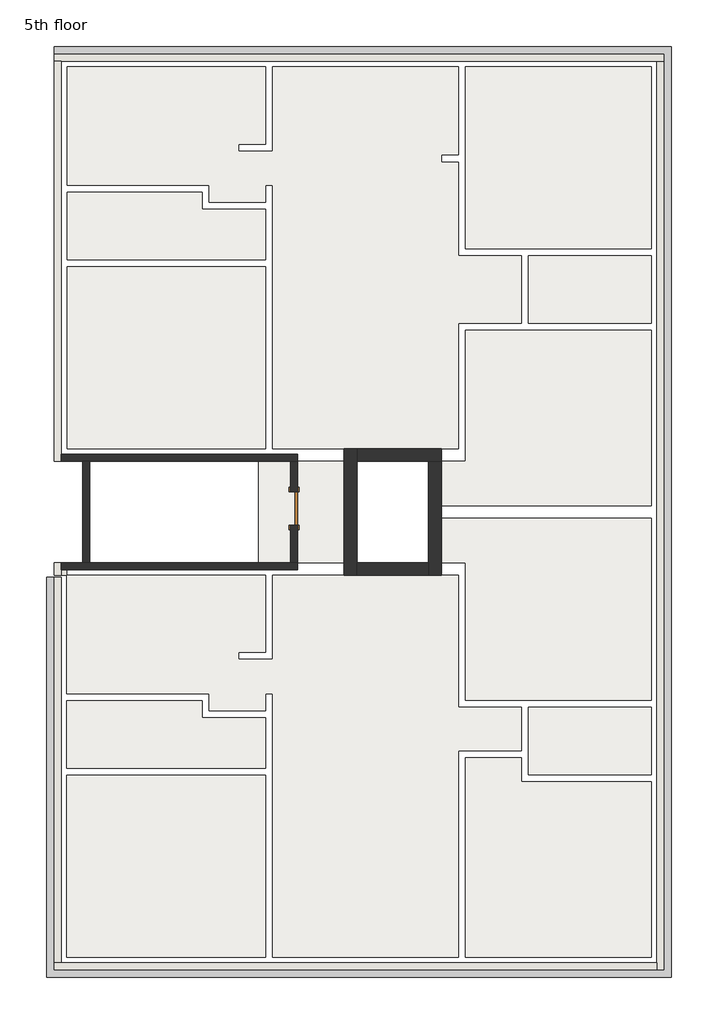
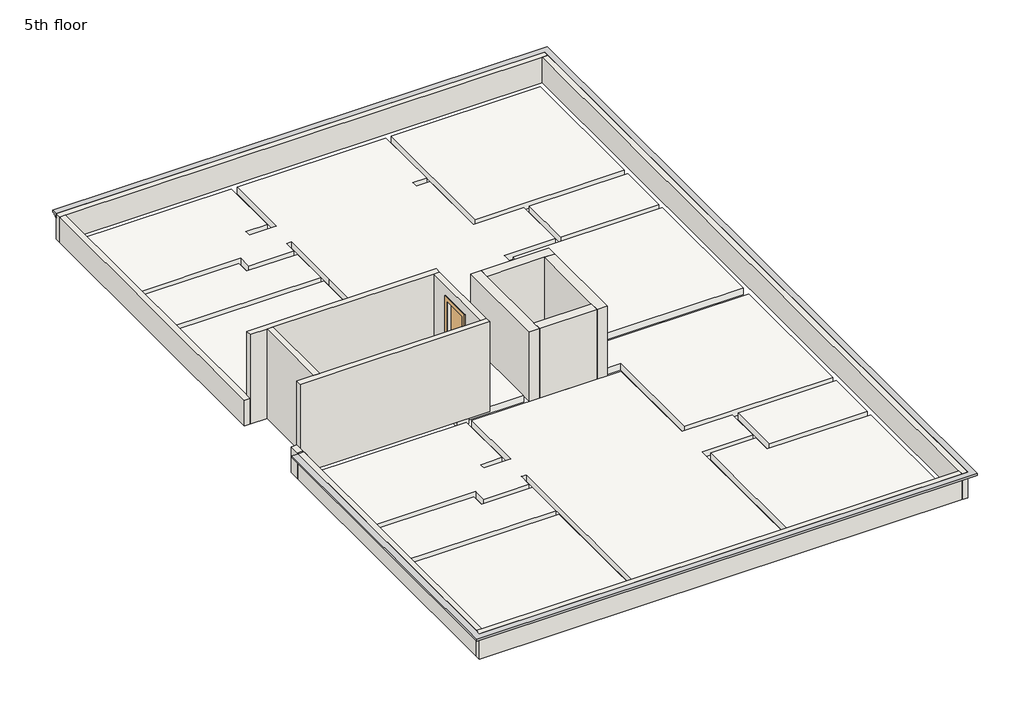
# One storey: 15 walls, 4 slabs, 1 door, 1 proxy.
"""IFC4 building model written with IfcOpenShell, lengths in millimetres."""

from ifc_helpers import new_model, si_unit, frame, origin, place, context, project, spatial, polyline, outline, extrude, faceted_brep, transform, mapped, element, save
from components import generic_models_46_generic_models_46_dc31fbd0, single_flush_2_x_7_door_01f1079d

model = new_model("IFC4")

# Units and contexts
model_context = context("Model", 3, world=origin())
ifc_project = project(units=[si_unit("LENGTHUNIT", "METRE", prefix="MILLI")], contexts=[model_context])

# Site, building, storey
site = spatial("IfcSite", under=ifc_project)
building = spatial("IfcBuilding", under=site)
storey = spatial("IfcBuildingStorey", under=building, Name="5th floor", Elevation=18288.0)

# Proxy
placement = place(None, origin())
generic_models_46_generic_models_46_shape = generic_models_46_generic_models_46_dc31fbd0(model_context)
element("IfcBuildingElementProxy", 1, Name="Generic Models 46 : Generic Models 46", ObjectType="Generic Models 46 : Generic Models 46", at=placement, inside=storey, context=model_context, shape_type="MappedRepresentation", body=[
    mapped(generic_models_46_generic_models_46_shape, transform((0.0, 0.0, 0.0), x_axis=(1.0, 0.0, 0.0), y_axis=(0.0, 1.0, 0.0), z_axis=(0.0, 0.0, 1.0))),
])

# Door
single_flush_2_x_7_door_shape = single_flush_2_x_7_door_01f1079d(model_context)
element("IfcDoor", 2, ObjectType="Single-Flush : 2' x 7' door", at=placement, inside=storey, context=model_context, shape_type="MappedRepresentation", body=[
    mapped(single_flush_2_x_7_door_shape, transform((-2101.8887202, 5079.7309003, 18288.0), x_axis=(0.0, -1.0, 0.0), y_axis=(1.0, 0.0, 0.0), z_axis=(0.0, 0.0, 1.0))),
])

# Slabs
element("IfcSlab", 3, ObjectType="FLOORING 6\"", at=placement, inside=storey, context=model_context, shape_type="SweptSolid", body=[
    extrude(outline(polyline([(4338.5987798, 13042.6309003), (4338.5987798, 9766.0309003), (985.7987798, 9766.0309003), (985.7987798, 13042.6309003), (4338.5987798, 13042.6309003)])), frame((0.0, 0.0, 18135.6), z_axis=(0.0, 0.0, 1.0), x_axis=(1.0, 0.0, 0.0)), (0.0, 0.0, 1.0), 152.4),
    extrude(outline(polyline([(4338.5987798, 9639.0309003), (4338.5987798, 8419.8309003), (2128.7987798, 8419.8309003), (2128.7987798, 9639.0309003), (4338.5987798, 9639.0309003)])), frame((0.0, 0.0, 18135.6), z_axis=(0.0, 0.0, 1.0), x_axis=(1.0, 0.0, 0.0)), (0.0, 0.0, 1.0), 152.4),
    extrude(outline(polyline([(-2621.0012202, 9435.8309003), (-2621.0012202, 6159.2309003), (-6202.4012202, 6159.2309003), (-6202.4012202, 9435.8309003), (-2621.0012202, 9435.8309003)])), frame((0.0, 0.0, 18135.6), z_axis=(0.0, 0.0, 1.0), x_axis=(1.0, 0.0, 0.0)), (0.0, 0.0, 1.0), 152.4),
    extrude(outline(polyline([(-2621.0012202, 9562.8309003), (-6202.4012202, 9562.8309003), (-6202.4012202, 10782.0309003), (-3764.0012202, 10782.0309003), (-3764.0012202, 10477.2309003), (-2621.0012202, 10477.2309003), (-2621.0012202, 9562.8309003)])), frame((0.0, 0.0, 18135.6), z_axis=(0.0, 0.0, 1.0), x_axis=(1.0, 0.0, 0.0)), (0.0, 0.0, 1.0), 152.4),
    extrude(outline(polyline([(553.9987798, 5930.6309003), (985.7987798, 5930.6309003), (985.7987798, 8292.8309003), (4338.5987798, 8292.8309003), (4338.5987798, 5130.5309003), (553.9987798, 5130.5309003), (553.9987798, 5930.6309003)])), frame((0.0, 0.0, 18135.6), z_axis=(0.0, 0.0, 1.0), x_axis=(1.0, 0.0, 0.0)), (0.0, 0.0, 1.0), 152.4),
])
element("IfcSlab", 4, ObjectType="FLOORING 6\"", at=placement, inside=storey, context=model_context, shape_type="SweptSolid", body=[
    extrude(outline(polyline([(985.7987798, 583.9309003), (2001.7987798, 583.9309003), (2001.7987798, 152.1309003), (4338.5987798, 152.1309003), (4338.5987798, -3010.1690997), (985.7987798, -3010.1690997), (985.7987798, 583.9309003)])), frame((0.0, 0.0, 18135.6), z_axis=(0.0, 0.0, 1.0), x_axis=(1.0, 0.0, 0.0)), (0.0, 0.0, 1.0), 152.4),
    extrude(outline(polyline([(-6203.9887202, -3010.1690997), (-6203.9887202, 266.4309003), (-2621.0012202, 266.4309003), (-2621.0012202, -3010.1690997), (-6203.9887202, -3010.1690997)])), frame((0.0, 0.0, 18135.6), z_axis=(0.0, 0.0, 1.0), x_axis=(1.0, 0.0, 0.0)), (0.0, 0.0, 1.0), 152.4),
    extrude(outline(polyline([(-2621.0012202, 393.4309003), (-6203.9887202, 393.4309003), (-6203.9887202, 1612.6309003), (-3764.0012202, 1612.6309003), (-3764.0012202, 1307.8309003), (-2621.0012202, 1307.8309003), (-2621.0012202, 393.4309003)])), frame((0.0, 0.0, 18135.6), z_axis=(0.0, 0.0, 1.0), x_axis=(1.0, 0.0, 0.0)), (0.0, 0.0, 1.0), 152.4),
    extrude(outline(polyline([(858.7987798, -3010.1690997), (-2494.0012202, -3010.1690997), (-2494.0012202, 1739.6309003), (-2621.0012202, 1739.6309003), (-2621.0012202, 1434.8309003), (-3637.0012202, 1434.8309003), (-3637.0012202, 1739.6309003), (-6203.9887202, 1739.6309003), (-6203.9887202, 3873.2309003), (-2621.0012202, 3873.2309003), (-2621.0012202, 2488.9309003), (-3103.6012202, 2488.9309003), (-3103.6012202, 2361.9309003), (-2494.0012202, 2361.9309003), (-2494.0012202, 3873.2309003), (858.7987798, 3873.2309003), (858.7987798, 1498.3309003), (2001.7987798, 1498.3309003), (2001.7987798, 710.9309003), (858.7987798, 710.9309003), (858.7987798, -3010.1690997)])), frame((0.0, 0.0, 18135.6), z_axis=(0.0, 0.0, 1.0), x_axis=(1.0, 0.0, 0.0)), (0.0, 0.0, 1.0), 152.4),
    extrude(outline(polyline([(985.7987798, 1625.3309003), (985.7987798, 4101.8309003), (553.9987798, 4101.8309003), (553.9987798, 4901.9309003), (4338.5987798, 4901.9309003), (4338.5987798, 1625.3309003), (985.7987798, 1625.3309003)])), frame((0.0, 0.0, 18135.6), z_axis=(0.0, 0.0, 1.0), x_axis=(1.0, 0.0, 0.0)), (0.0, 0.0, 1.0), 152.4),
    extrude(outline(polyline([(-2748.0012202, 4000.2309003), (-2748.0012202, 5981.4309003), (-2748.0012202, 6032.2309003), (-2494.0012202, 6032.2309003), (-2494.0012202, 5930.6309003), (-1198.6012202, 5930.6309003), (-1198.6012202, 4101.8309003), (-2494.0012202, 4101.8309003), (-2494.0012202, 4000.2309003), (-2748.0012202, 4000.2309003)])), frame((0.0, 0.0, 18135.6), z_axis=(0.0, 0.0, 1.0), x_axis=(1.0, 0.0, 0.0)), (0.0, 0.0, 1.0), 152.4),
])
element("IfcSlab", 5, ObjectType="FLOORING 6\"", at=placement, inside=storey, context=model_context, shape_type="SweptSolid", body=[
    extrude(outline(polyline([(-2621.0012202, 11645.6309003), (-3103.6012202, 11645.6309003), (-3103.6012202, 11518.6309003), (-2557.5012202, 11518.6309003), (-2494.0012202, 11518.6309003), (-2494.0012202, 13042.6309003), (858.7987798, 13042.6309003), (858.7987798, 11455.1309003), (553.9987798, 11455.1309003), (553.9987798, 11328.1309003), (858.7987798, 11328.1309003), (858.7987798, 9639.0309003), (2001.7987798, 9639.0309003), (2001.7987798, 8419.8309003), (858.7987798, 8419.8309003), (858.7987798, 6159.2309003), (-2494.0012202, 6159.2309003), (-2494.0012202, 9435.8309003), (-2494.0012202, 10909.0309003), (-2621.0012202, 10909.0309003), (-2621.0012202, 10604.2309003), (-3637.0012202, 10604.2309003), (-3637.0012202, 10909.0309003), (-6202.4012202, 10909.0309003), (-6202.4012202, 13042.6309003), (-2621.0012202, 13042.6309003), (-2621.0012202, 11645.6309003)])), frame((0.0, 0.0, 18135.6), z_axis=(0.0, 0.0, 1.0), x_axis=(1.0, 0.0, 0.0)), (0.0, 0.0, 1.0), 152.4),
])
element("IfcSlab", 6, ObjectType="bathroom tiles", at=placement, inside=storey, context=model_context, shape_type="SweptSolid", body=[
    extrude(outline(polyline([(4338.5987798, 1498.3309003), (4338.5987798, 279.1309003), (2128.7987798, 279.1309003), (2128.7987798, 1498.3309003), (4338.5987798, 1498.3309003)])), frame((0.0, 0.0, 18135.6), z_axis=(0.0, 0.0, 1.0), x_axis=(1.0, 0.0, 0.0)), (0.0, 0.0, 1.0), 152.4),
])

# Walls
element("IfcWall", 7, ObjectType="OUTER WALL 9\"", at=placement, inside=storey, context=model_context, shape_type="Brep", body=[
    faceted_brep([(-970.0012202, 3873.2309003, 18288.0), (-970.0012202, 4101.8309003, 18288.0), (-970.0012202, 5930.6309003, 18288.0), (-970.0012202, 6159.2309003, 18288.0), (-970.0012202, 6159.2309003, 19943.9320422), (-970.0012202, 5930.6309003, 19943.9320422), (-970.0012202, 4101.8309003, 19943.9320422), (-970.0012202, 3873.2309003, 19943.9320422), (-1198.6012202, 3873.2309003, 18288.0), (-1198.6012202, 3873.2309003, 19943.9320422), (-1198.6012202, 6159.2309003, 19943.9320422), (-1198.6012202, 6159.2309003, 18288.0)], [[[0, 1, 2, 3, 4, 5, 6, 7]], [[8, 9, 10, 11]], [[3, 2, 1, 0, 8, 11]], [[7, 6, 5, 4, 10, 9]], [[4, 3, 11, 10]], [[0, 7, 9, 8]]]),
])
element("IfcWall", 8, ObjectType="OUTER WALL 9\"", at=placement, inside=storey, context=model_context, shape_type="Brep", body=[
    faceted_brep([(-970.0012202, 5930.6309003, 18288.0), (325.3987798, 5930.6309003, 18288.0), (553.9987798, 5930.6309003, 18288.0), (553.9987798, 5930.6309003, 19943.9320422), (325.3987798, 5930.6309003, 19943.9320422), (-970.0012202, 5930.6309003, 19943.9320422), (-970.0012202, 6159.2309003, 18288.0), (-970.0012202, 6159.2309003, 19943.9320422), (553.9987798, 6159.2309003, 19943.9320422), (553.9987798, 6159.2309003, 18288.0)], [[[0, 1, 2, 3, 4, 5]], [[6, 7, 8, 9]], [[2, 1, 0, 6, 9]], [[5, 4, 3, 8, 7]], [[0, 5, 7, 6]], [[3, 2, 9, 8]]]),
])
element("IfcWall", 9, ObjectType="OUTER WALL 9\"", at=placement, inside=storey, context=model_context, shape_type="Brep", body=[
    faceted_brep([(325.3987798, 5930.6309003, 18288.0), (325.3987798, 4101.8309003, 18288.0), (325.3987798, 3873.2309003, 18288.0), (325.3987798, 3873.2309003, 19943.9320422), (325.3987798, 4101.8309003, 19943.9320422), (325.3987798, 5930.6309003, 19943.9320422), (553.9987798, 5930.6309003, 18288.0), (553.9987798, 5930.6309003, 19943.9320422), (553.9987798, 3873.2309003, 19943.9320422), (553.9987798, 3873.2309003, 18288.0)], [[[0, 1, 2, 3, 4, 5]], [[6, 7, 8, 9]], [[2, 1, 0, 6, 9]], [[5, 4, 3, 8, 7]], [[0, 5, 7, 6]], [[3, 2, 9, 8]]]),
])
element("IfcWall", 10, ObjectType="OUTER WALL 9\"", at=placement, inside=storey, context=model_context, shape_type="SweptSolid", body=[
    extrude(outline(polyline([(-970.0012202, 4101.8309003), (325.3987798, 4101.8309003), (325.3987798, 3873.2309003), (-970.0012202, 3873.2309003), (-970.0012202, 4101.8309003)])), frame((0.0, 0.0, 18288.0), z_axis=(0.0, 0.0, 1.0), x_axis=(1.0, 0.0, 0.0)), (0.0, 0.0, 1.0), 1655.9320422),
])
element("IfcWall", 11, ObjectType="inner wall 5\"", at=placement, inside=storey, context=model_context, shape_type="Brep", body=[
    faceted_brep([(-6432.5887202, 13144.2309003, 18288.0), (-6305.5887202, 13144.2309003, 18288.0), (4440.1987798, 13144.2309003, 18288.0), (4567.1987798, 13144.2309003, 18288.0), (4567.1987798, 13144.2309003, 18897.6), (4440.1987798, 13144.2309003, 18897.6), (-6305.5887202, 13144.2309003, 18897.6), (-6432.5887202, 13144.2309003, 18897.6), (-6432.5887202, 13271.2309003, 18288.0), (-6432.5887202, 13271.2309003, 18897.6), (4567.1987798, 13271.2309003, 18897.6), (4567.1987798, 13271.2309003, 18288.0)], [[[0, 1, 2, 3, 4, 5, 6, 7]], [[8, 9, 10, 11]], [[3, 2, 1, 0, 8, 11]], [[7, 6, 5, 4, 10, 9]], [[4, 3, 11, 10]], [[0, 7, 9, 8]]]),
])
element("IfcWall", 12, ObjectType="inner wall 5\"", at=placement, inside=storey, context=model_context, shape_type="Brep", body=[
    faceted_brep([(4440.1987798, 13144.2309003, 18288.0), (4440.1987798, -3111.7690997, 18288.0), (4440.1987798, -3238.7690997, 18288.0), (4440.1987798, -3238.7690997, 18897.6), (4440.1987798, -3111.7690997, 18897.6), (4440.1987798, 13144.2309003, 18897.6), (4567.1987798, 13144.2309003, 18288.0), (4567.1987798, 13144.2309003, 18897.6), (4567.1987798, -3238.7690997, 18897.6), (4567.1987798, -3238.7690997, 18288.0)], [[[0, 1, 2, 3, 4, 5]], [[6, 7, 8, 9]], [[2, 1, 0, 6, 9]], [[5, 4, 3, 8, 7]], [[0, 5, 7, 6]], [[3, 2, 9, 8]]]),
])
element("IfcWall", 13, ObjectType="inner wall 5\"", at=placement, inside=storey, context=model_context, shape_type="Brep", body=[
    faceted_brep([(4440.1987798, -3111.7690997, 18288.0), (-6305.5887202, -3111.7690997, 18288.0), (-6432.5887202, -3111.7690997, 18288.0), (-6432.5887202, -3111.7690997, 18897.6), (-6305.5887202, -3111.7690997, 18897.6), (4440.1987798, -3111.7690997, 18897.6), (4440.1987798, -3238.7690997, 18288.0), (4440.1987798, -3238.7690997, 18897.6), (-6432.5887202, -3238.7690997, 18897.6), (-6432.5887202, -3238.7690997, 18288.0)], [[[0, 1, 2, 3, 4, 5]], [[6, 7, 8, 9]], [[2, 1, 0, 6, 9]], [[5, 4, 3, 8, 7]], [[0, 5, 7, 6]], [[3, 2, 9, 8]]]),
])
element("IfcWall", 14, ObjectType="inner wall 5\"", at=placement, inside=storey, context=model_context, shape_type="SweptSolid", body=[
    extrude(outline(polyline([(-6305.5887202, 3835.1309003), (-6305.5887202, -3111.7690997), (-6432.5887202, -3111.7690997), (-6432.5887202, 3835.1309003), (-6305.5887202, 3835.1309003)])), frame((0.0, 0.0, 18288.0), z_axis=(0.0, 0.0, 1.0), x_axis=(1.0, 0.0, 0.0)), (0.0, 0.0, 1.0), 609.6),
])
element("IfcWall", 15, ObjectType="inner wall 5\"", at=placement, inside=storey, context=model_context, shape_type="Brep", body=[
    faceted_brep([(-6432.5887202, 13144.2309003, 18288.0), (-6432.5887202, 5930.6309003, 18288.0), (-6432.5887202, 5930.6309003, 18897.6), (-6432.5887202, 13144.2309003, 18897.6), (-6305.5887202, 13144.2309003, 18288.0), (-6305.5887202, 13144.2309003, 18897.6), (-6305.5887202, 5930.6309003, 18897.6), (-6305.5887202, 5930.6309003, 18288.0), (-6305.5887202, 6057.6309003, 18288.0)], [[[0, 1, 2, 3]], [[4, 5, 6, 7, 8]], [[1, 0, 4, 8, 7]], [[3, 2, 6, 5]], [[2, 1, 7, 6]], [[0, 3, 5, 4]]]),
])
element("IfcWall", 16, ObjectType="inner wall 5\"", at=placement, inside=storey, context=model_context, shape_type="Brep", body=[
    faceted_brep([(-6305.5887202, 5930.6309003, 18288.0), (-5923.0012202, 5930.6309003, 18288.0), (-5796.0012202, 5930.6309003, 18288.0), (-2165.3887202, 5930.6309003, 18288.0), (-2038.3887202, 5930.6309003, 18288.0), (-2038.3887202, 5930.6309003, 20421.6), (-2165.3887202, 5930.6309003, 20421.6), (-5796.0012202, 5930.6309003, 20421.6), (-5923.0012202, 5930.6309003, 20421.6), (-6305.5887202, 5930.6309003, 20421.6), (-6305.5887202, 5930.6309003, 18897.6), (-6305.5887202, 6057.6309003, 18288.0), (-6305.5887202, 6057.6309003, 20421.6), (-2038.3887202, 6057.6309003, 20421.6), (-2038.3887202, 6057.6309003, 18288.0)], [[[0, 1, 2, 3, 4, 5, 6, 7, 8, 9, 10]], [[11, 12, 13, 14]], [[4, 3, 2, 1, 0, 11, 14]], [[5, 4, 14, 13]], [[9, 8, 7, 6, 5, 13, 12]], [[0, 10, 9, 12, 11]]]),
])
element("IfcWall", 17, ObjectType="inner wall 5\"", at=placement, inside=storey, context=model_context, shape_type="SweptSolid", body=[
    extrude(outline(polyline([(-5923.0012202, 4101.8309003), (-5923.0012202, 5930.6309003), (-5796.0012202, 5930.6309003), (-5796.0012202, 4101.8309003), (-5923.0012202, 4101.8309003)])), frame((0.0, 0.0, 18288.0), z_axis=(0.0, 0.0, 1.0), x_axis=(1.0, 0.0, 0.0)), (0.0, 0.0, 1.0), 2133.6),
])
element("IfcWall", 18, ObjectType="inner wall 5\"", at=placement, inside=storey, context=model_context, shape_type="Brep", body=[
    faceted_brep([(-2038.3887202, 4101.6567318, 18288.0), (-2165.3887202, 4101.6567318, 18288.0), (-6305.5887202, 4101.6567318, 18288.0), (-6305.5887202, 4101.6567318, 18897.6), (-6305.5887202, 4101.6567318, 20421.6), (-2165.3887202, 4101.6567318, 20421.6), (-2038.3887202, 4101.6567318, 20421.6), (-2038.3887202, 3974.6567318, 18288.0), (-2038.3887202, 3974.6567318, 20421.6), (-6305.5887202, 3974.6567318, 20421.6), (-6305.5887202, 3974.6567318, 18288.0)], [[[0, 1, 2, 3, 4, 5, 6]], [[7, 8, 9, 10]], [[2, 1, 0, 7, 10]], [[6, 5, 4, 9, 8]], [[4, 3, 2, 10, 9]], [[0, 6, 8, 7]]]),
])
element("IfcWall", 19, ObjectType="inner wall 5\"", at=placement, inside=storey, context=model_context, shape_type="Brep", body=[
    faceted_brep([(-6432.5887202, 4101.6567318, 18288.0), (-6432.5887202, 3873.2309003, 18288.0), (-6432.5887202, 3873.2309003, 18897.6), (-6432.5887202, 4101.6567318, 18897.6), (-6305.5887202, 4101.6567318, 18288.0), (-6305.5887202, 4101.6567318, 18897.6), (-6305.5887202, 3873.2309003, 18897.6), (-6305.5887202, 3873.2309003, 18764.4643868), (-6305.5887202, 3873.2309003, 18288.0), (-6305.5887202, 3974.6567318, 18288.0), (-6305.5887202, 4000.2309003, 18288.0)], [[[0, 1, 2, 3]], [[4, 5, 6, 7, 8, 9, 10]], [[1, 0, 4, 10, 9, 8]], [[3, 2, 6, 5]], [[0, 3, 5, 4]], [[2, 1, 8, 7, 6]]]),
])
element("IfcWall", 20, ObjectType="inner wall 5\"", at=placement, inside=storey, context=model_context, shape_type="SweptSolid", body=[
    extrude(outline(polyline([(-6203.9887202, 3873.2309003), (-6305.5887202, 3873.2309003), (-6305.5887202, 4000.2309003), (-6203.9887202, 4000.2309003), (-6203.9887202, 3873.2309003)])), frame((0.0, 0.0, 18288.0), z_axis=(0.0, 0.0, 1.0), x_axis=(1.0, 0.0, 0.0)), (0.0, 0.0, 1.0), 476.4643868),
])
element("IfcWall", 21, ObjectType="inner wall 5\"", at=placement, inside=storey, context=model_context, shape_type="SweptSolid", body=[
    extrude(outline(polyline([(4101.6567318, 20421.6), (5930.6309003, 20421.6), (5930.6309003, 18288.0), (5384.5309003, 18288.0), (5384.5309003, 20116.8), (4774.9309003, 20116.8), (4774.9309003, 18288.0), (4101.6567318, 18288.0), (4101.6567318, 20421.6)])), frame((-2165.3887202, 0.0, 0.0), z_axis=(1.0, 0.0, 0.0), x_axis=(0.0, 1.0, 0.0)), (0.0, 0.0, 1.0), 127.0),
])

save(model, "model.ifc")

# Revit data of these elements
# Type "Single-Flush : 2' x 7' door"
#   Type Mark = "18"
#   Construction Type Id = "MDOOR"
#   Assembly Code = "C1020"
#   Analytic Construction = "Metal"
#   Thickness = 0' - 2"
#   Heat Transfer Coefficient (U) = 0.651978 BTU/(h·ft²·°F)
#   Height = 6' - 0"
#   Trim Projection Ext = 0' - 1"
#   Trim Projection Int = 0' - 1"
#   Trim Width = 0' - 3"
#   Width = 2' - 0"
#   Define Thermal Properties by = 1
#   Door Material = Door - Panel
#   Frame Material = Door - Frame
#   Visual Light Transmittance = 0
#   Solar Heat Gain Coefficient = 0
#   Function = (empty or 0)
#   Wall Closure = (empty or 0)
# Type "FLOORING 6\""
#   Assembly Code = "B1010"
#   Function = 0
#   Layers, outside or top first: 0' - 6" "MARBLE FLOORING" (function 1)
# Type "bathroom tiles"
#   Assembly Code = "B1010"
#   Function = 0
#   Layers, outside or top first: 0' - 6" "tile flooring" (function 1)
# Type "OUTER WALL 9\""
#   Assembly Code = "B2010"
#   Layers, outside or top first: 0' - 9" "ROSE COLOUR" (function 1)
# Type "inner wall 5\""
#   Assembly Code = "B2010"
#   Layers, outside or top first: 0' - 5" "ROSE COLOUR" (function 1)
# Element 1 (IfcBuildingElementProxy, "Generic Models 46 : Generic Models 46")
#   Phase Created = New Construction
#   Materials on its faces: "white"
# Element 2 (IfcDoor, "Single-Flush : 2' x 7' door")
#   Phase Created = New Construction
#   Materials on its faces: "Door - Frame", "Door - Panel"
# Element 3 (IfcSlab, "FLOORING 6\"")
#   Height Offset From Level = 0' - 0"
#   Phase Created = New Construction
#   Materials on its faces: "MARBLE FLOORING"
# Element 4 (IfcSlab, "FLOORING 6\"")
#   built-in parameter 1001955 = 1.5708 (stored number, unit not read)
#   Height Offset From Level = 0' - 0"
#   Phase Created = New Construction
#   Materials on its faces: "MARBLE FLOORING"
# Element 5 (IfcSlab, "FLOORING 6\"")
#   built-in parameter 1001955 = -1.5708 (stored number, unit not read)
#   Height Offset From Level = 0' - 0"
#   Phase Created = New Construction
#   Materials on its faces: "MARBLE FLOORING"
# Element 6 (IfcSlab, "bathroom tiles")
#   Height Offset From Level = 0' - 0"
#   Phase Created = New Construction
#   Materials on its faces: "tile flooring"
# Elements 7, 8, 9, 10 (IfcWall, "OUTER WALL 9\"")
#   Top Offset = -1' - 6.80583"
#   Base Offset = 0' - 0"
#   wall height = 5' - 5.19417"
#   Phase Created = New Construction
#   Base Constraint = 5th floor
#   Top Constraint = TOP OF ROOF
#   Materials on its faces: "ROSE COLOUR"
# Elements 11, 12, 13, 14, 15, 19 (IfcWall, "inner wall 5\"")
#   Top Offset = 0' - 0"
#   Base Offset = 0' - 0"
#   Unconnected Height = 2' - 0"
#   wall height = 2' - 0"
#   Phase Created = New Construction
#   Base Constraint = 5th floor
#   Materials on its faces: "ROSE COLOUR"
# Elements 16, 21 (IfcWall, "inner wall 5\"")
#   Top Offset = 0' - 0"
#   Base Offset = 0' - 0"
#   wall height = 7' - 0"
#   Phase Created = New Construction
#   Base Constraint = 5th floor
#   Top Constraint = TOP OF ROOF
#   Materials on its faces: "ROSE COLOUR"
# Elements 17, 18 (IfcWall, "inner wall 5\"")
#   Top Offset = 0' - 0"
#   Base Offset = 0' - 0"
#   Unconnected Height = 7' - 0"
#   wall height = 7' - 0"
#   Phase Created = New Construction
#   Base Constraint = 5th floor
#   Materials on its faces: "ROSE COLOUR"
# Element 20 (IfcWall, "inner wall 5\"")
#   Top Offset = -5' - 5.24156"
#   Base Offset = 0' - 0"
#   wall height = 1' - 6.75844"
#   Phase Created = New Construction
#   Base Constraint = 5th floor
#   Top Constraint = TOP OF ROOF
#   Materials on its faces: "ROSE COLOUR"
# Materials
#   "Door - Panel": class "Wood", colour RGB 210 159 95, transparency 0, Cost = 0
#   "Door - Frame": colour RGB 118 70 51, transparency 0, Cost = 0
#   "MARBLE FLOORING": class "Generic", colour RGB 120 120 120, transparency 0, Cost = 0
#   "tile flooring": class "Generic", colour RGB 120 120 120, transparency 0, Cost = 0
#   "ROSE COLOUR": class "Generic", colour RGB 120 120 120, transparency 0, Cost = 0
#   "white": class "Generic", colour RGB 120 120 120, transparency 0, Cost = 0
